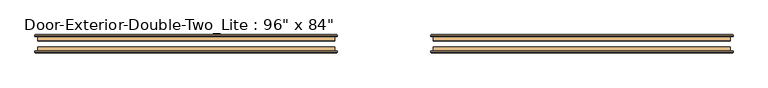
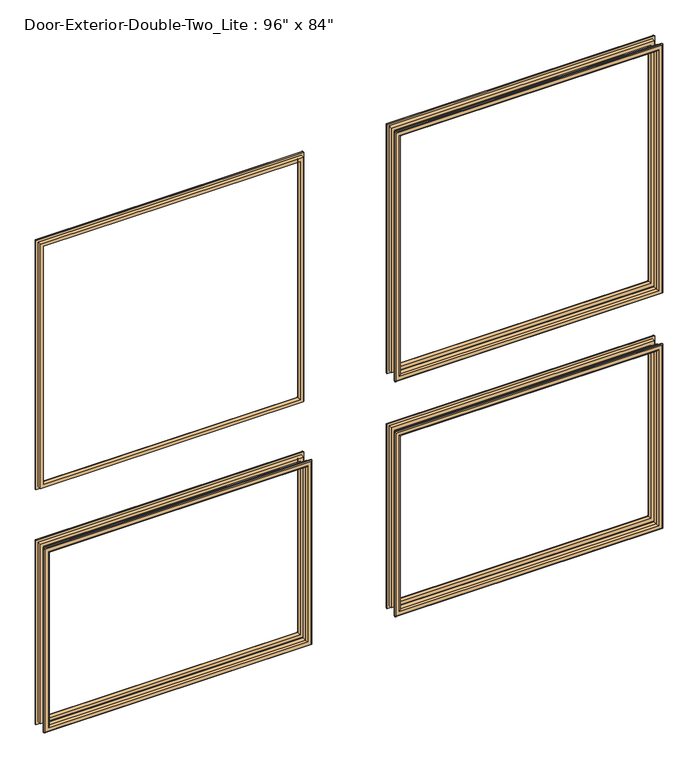
"""IFC4 building model written with IfcOpenShell, lengths in millimetres: door geometry."""

from ifc_helpers import new_model, si_unit, frame, origin, place, context, project, spatial, ellipse_curve, source, transform, mapped, element, save
from ifc_brep_helpers import plane_surface, cylinder_surface, advanced_brep


def door_142f3e8c(model_context):
    return source(origin(), model_context, "Body", "AdvancedBrep", [
        advanced_brep(
        [(-1066.8, 69.85, 914.4), (-1066.8, 82.55, 914.4), (-1066.8, 82.55, 254.0), (-1066.8, 69.85, 254.0), (-1054.8, 83.55, 902.4), (-1054.8, 69.85, 902.4), (-1054.8, 69.85, 266.0), (-1054.8, 83.55, 266.0), (-1059.8, 88.55, 907.4), (-1059.8, 88.55, 261.0), (-1074.8, 86.55, 922.4), (-1072.8, 88.55, 920.4), (-1072.8, 88.55, 248.0), (-1074.8, 86.55, 246.0), (-1074.8, 82.55, 922.4), (-1074.8, 82.55, 246.0), (-152.4, 82.55, 254.0), (-152.4, 69.85, 254.0), (-164.4, 69.85, 266.0), (-164.4, 83.55, 266.0), (-159.4, 88.55, 261.0), (-146.4, 88.55, 248.0), (-144.4, 86.55, 246.0), (-144.4, 82.55, 246.0), (-152.4, 82.55, 914.4), (-152.4, 69.85, 914.4), (-164.4, 69.85, 902.4), (-164.4, 83.55, 902.4), (-159.4, 88.55, 907.4), (-146.4, 88.55, 920.4), (-144.4, 86.55, 922.4), (-144.4, 82.55, 922.4)],
        [
            (0, 1),
            (1, 2),
            (2, 3),
            (3, 0),
            (4, 5),
            (5, 6),
            (6, 7),
            (7, 4),
            (8, 4, ellipse_curve(frame((-1059.8, 83.55, 907.4), z_axis=(-0.7071067811865475, 0.0, -0.7071067811865475), x_axis=(-0.7071067811865474, 0.0, 0.7071067811865476)), 7.0710678, 5.0)),
            (7, 9, ellipse_curve(frame((-1059.8, 83.55, 261.0), z_axis=(-0.7071067811865475, 0.0, 0.7071067811865475), x_axis=(0.7071067811865474, 0.0, 0.7071067811865476)), 7.0710678, 5.0)),
            (9, 8),
            (10, 11, ellipse_curve(frame((-1072.8, 86.55, 920.4), z_axis=(-0.7071067811865475, 0.0, -0.7071067811865475), x_axis=(-0.7071067811865474, 0.0, 0.7071067811865476)), 2.8284271, 2.0)),
            (11, 12),
            (12, 13, ellipse_curve(frame((-1072.8, 86.55, 248.0), z_axis=(-0.7071067811865475, 0.0, 0.7071067811865475), x_axis=(0.7071067811865474, 0.0, 0.7071067811865476)), 2.8284271, 2.0)),
            (13, 10),
            (14, 10),
            (13, 15),
            (15, 14),
            (2, 16),
            (16, 17),
            (17, 3),
            (6, 18),
            (18, 19),
            (19, 7),
            (19, 20, ellipse_curve(frame((-159.4, 83.55, 261.0), z_axis=(-0.7071067811865475, 0.0, -0.7071067811865475), x_axis=(-0.7071067811865476, 0.0, 0.7071067811865474)), 7.0710678, 5.0)),
            (20, 9),
            (12, 21),
            (21, 22, ellipse_curve(frame((-146.4, 86.55, 248.0), z_axis=(-0.7071067811865475, 0.0, -0.7071067811865475), x_axis=(-0.7071067811865476, 0.0, 0.7071067811865474)), 2.8284271, 2.0)),
            (22, 13),
            (22, 23),
            (23, 15),
            (16, 24),
            (24, 25),
            (25, 17),
            (18, 26),
            (26, 27),
            (27, 19),
            (27, 28, ellipse_curve(frame((-159.4, 83.55, 907.4), z_axis=(0.7071067811865475, 0.0, -0.7071067811865475), x_axis=(-0.7071067811865474, 0.0, -0.7071067811865476)), 7.0710678, 5.0)),
            (28, 20),
            (21, 29),
            (29, 30, ellipse_curve(frame((-146.4, 86.55, 920.4), z_axis=(0.7071067811865475, 0.0, -0.7071067811865475), x_axis=(-0.7071067811865474, 0.0, -0.7071067811865476)), 2.8284271, 2.0)),
            (30, 22),
            (30, 31),
            (31, 23),
            (31, 14),
            (1, 24),
            (0, 25),
            (5, 26),
            (4, 27),
            (8, 28),
            (11, 29),
            (10, 30),
        ],
        [
            plane_surface(frame((-1066.8, 82.55, 914.4), z_axis=(-1.0, 0.0, 0.0), x_axis=(0.0, 0.0, -1.0))),
            plane_surface(frame((-1054.8, 69.85, 902.4), z_axis=(1.0, 0.0, 0.0), x_axis=(0.0, 0.0, -1.0))),
            cylinder_surface(frame((-1059.8, 83.55, 914.4), z_axis=(0.0, 0.0, 1.0), x_axis=(-1.0, 0.0, 0.0)), 5.0),
            cylinder_surface(frame((-1072.8, 86.55, 914.4), z_axis=(0.0, 0.0, 1.0), x_axis=(-1.0, 0.0, 0.0)), 2.0),
            plane_surface(frame((-1074.8, 86.55, 922.4), z_axis=(-1.0, 0.0, 0.0), x_axis=(0.0, 0.0, -1.0))),
            plane_surface(frame((-1066.8, 82.55, 254.0), z_axis=(0.0, 0.0, -1.0), x_axis=(1.0, 0.0, 0.0))),
            plane_surface(frame((-1054.8, 69.85, 266.0), z_axis=(0.0, 0.0, 1.0), x_axis=(1.0, 0.0, 0.0))),
            cylinder_surface(frame((-1066.8, 83.55, 261.0), z_axis=(-1.0, 0.0, 0.0), x_axis=(0.0, 0.0, -1.0)), 5.0),
            cylinder_surface(frame((-1066.8, 86.55, 248.0), z_axis=(-1.0, 0.0, 0.0), x_axis=(0.0, 0.0, -1.0)), 2.0),
            plane_surface(frame((-1074.8, 86.55, 246.0), z_axis=(0.0, 0.0, -1.0), x_axis=(1.0, 0.0, 0.0))),
            plane_surface(frame((-152.4, 82.55, 254.0), z_axis=(1.0, 0.0, 0.0), x_axis=(0.0, 0.0, 1.0))),
            plane_surface(frame((-164.4, 69.85, 266.0), z_axis=(-1.0, 0.0, 0.0), x_axis=(0.0, 0.0, 1.0))),
            cylinder_surface(frame((-159.4, 83.55, 254.0), z_axis=(0.0, 0.0, -1.0), x_axis=(1.0, 0.0, 0.0)), 5.0),
            cylinder_surface(frame((-146.4, 86.55, 254.0), z_axis=(0.0, 0.0, -1.0), x_axis=(1.0, 0.0, 0.0)), 2.0),
            plane_surface(frame((-144.4, 86.55, 246.0), z_axis=(1.0, 0.0, 0.0), x_axis=(0.0, 0.0, 1.0))),
            plane_surface(frame((-144.4, 82.55, 922.4), z_axis=(0.0, -1.0, 0.0), x_axis=(-1.0, 0.0, 0.0))),
            plane_surface(frame((-152.4, 82.55, 914.4), z_axis=(0.0, 0.0, 1.0), x_axis=(-1.0, 0.0, 0.0))),
            plane_surface(frame((-152.4, 69.85, 914.4), z_axis=(0.0, -1.0, 0.0), x_axis=(-1.0, 0.0, 0.0))),
            plane_surface(frame((-164.4, 69.85, 902.4), z_axis=(0.0, 0.0, -1.0), x_axis=(-1.0, 0.0, 0.0))),
            cylinder_surface(frame((-152.4, 83.55, 907.4), z_axis=(1.0, 0.0, 0.0), x_axis=(0.0, 0.0, 1.0)), 5.0),
            plane_surface(frame((-159.4, 88.55, 907.4), z_axis=(0.0, 1.0, 0.0), x_axis=(-1.0, 0.0, 0.0))),
            cylinder_surface(frame((-152.4, 86.55, 920.4), z_axis=(1.0, 0.0, 0.0), x_axis=(0.0, 0.0, 1.0)), 2.0),
            plane_surface(frame((-144.4, 86.55, 922.4), z_axis=(0.0, 0.0, 1.0), x_axis=(-1.0, 0.0, 0.0))),
        ],
        [
            (0, [[1, 2, 3, 4]]),
            (1, [[5, 6, 7, 8]]),
            (2, [[9, -8, 10, 11]]),
            (3, [[12, 13, 14, 15]]),
            (4, [[16, -15, 17, 18]]),
            (5, [[-3, 19, 20, 21]]),
            (6, [[-7, 22, 23, 24]]),
            (7, [[-10, -24, 25, 26]]),
            (8, [[-14, 27, 28, 29]]),
            (9, [[-17, -29, 30, 31]]),
            (10, [[-20, 32, 33, 34]]),
            (11, [[-23, 35, 36, 37]]),
            (12, [[-25, -37, 38, 39]]),
            (13, [[-28, 40, 41, 42]]),
            (14, [[-30, -42, 43, 44]]),
            (15, [[-31, -44, 45, -18], [46, -32, -19, -2]]),
            (16, [[-33, -46, -1, 47]]),
            (17, [[-21, -34, -47, -4], [48, -35, -22, -6]]),
            (18, [[-36, -48, -5, 49]]),
            (19, [[-38, -49, -9, 50]]),
            (20, [[51, -40, -27, -13], [-26, -39, -50, -11]]),
            (21, [[-41, -51, -12, 52]]),
            (22, [[-43, -52, -16, -45]]),
        ],
    ),
        advanced_brep(
        [(152.4, 69.85, 914.4), (152.4, 82.55, 914.4), (152.4, 82.55, 254.0), (152.4, 69.85, 254.0), (164.4, 83.55, 902.4), (164.4, 69.85, 902.4), (164.4, 69.85, 266.0), (164.4, 83.55, 266.0), (159.4, 88.55, 907.4), (159.4, 88.55, 261.0), (144.4, 86.55, 922.4), (146.4, 88.55, 920.4), (146.4, 88.55, 248.0), (144.4, 86.55, 246.0), (144.4, 82.55, 922.4), (144.4, 82.55, 246.0), (1066.8, 82.55, 254.0), (1066.8, 69.85, 254.0), (1054.8, 69.85, 266.0), (1054.8, 83.55, 266.0), (1059.8, 88.55, 261.0), (1072.8, 88.55, 248.0), (1074.8, 86.55, 246.0), (1074.8, 82.55, 246.0), (1066.8, 82.55, 914.4), (1066.8, 69.85, 914.4), (1054.8, 69.85, 902.4), (1054.8, 83.55, 902.4), (1059.8, 88.55, 907.4), (1072.8, 88.55, 920.4), (1074.8, 86.55, 922.4), (1074.8, 82.55, 922.4)],
        [
            (0, 1),
            (1, 2),
            (2, 3),
            (3, 0),
            (4, 5),
            (5, 6),
            (6, 7),
            (7, 4),
            (8, 4, ellipse_curve(frame((159.4, 83.55, 907.4), z_axis=(-0.7071067811865475, 0.0, -0.7071067811865475), x_axis=(-0.7071067811865474, 0.0, 0.7071067811865476)), 7.0710678, 5.0)),
            (7, 9, ellipse_curve(frame((159.4, 83.55, 261.0), z_axis=(-0.7071067811865475, 0.0, 0.7071067811865475), x_axis=(0.7071067811865474, 0.0, 0.7071067811865476)), 7.0710678, 5.0)),
            (9, 8),
            (10, 11, ellipse_curve(frame((146.4, 86.55, 920.4), z_axis=(-0.7071067811865475, 0.0, -0.7071067811865475), x_axis=(-0.7071067811865474, 0.0, 0.7071067811865476)), 2.8284271, 2.0)),
            (11, 12),
            (12, 13, ellipse_curve(frame((146.4, 86.55, 248.0), z_axis=(-0.7071067811865475, 0.0, 0.7071067811865475), x_axis=(0.7071067811865474, 0.0, 0.7071067811865476)), 2.8284271, 2.0)),
            (13, 10),
            (14, 10),
            (13, 15),
            (15, 14),
            (2, 16),
            (16, 17),
            (17, 3),
            (6, 18),
            (18, 19),
            (19, 7),
            (19, 20, ellipse_curve(frame((1059.8, 83.55, 261.0), z_axis=(-0.7071067811865475, 0.0, -0.7071067811865475), x_axis=(-0.7071067811865476, 0.0, 0.7071067811865474)), 7.0710678, 5.0)),
            (20, 9),
            (12, 21),
            (21, 22, ellipse_curve(frame((1072.8, 86.55, 248.0), z_axis=(-0.7071067811865475, 0.0, -0.7071067811865475), x_axis=(-0.7071067811865476, 0.0, 0.7071067811865474)), 2.8284271, 2.0)),
            (22, 13),
            (22, 23),
            (23, 15),
            (16, 24),
            (24, 25),
            (25, 17),
            (18, 26),
            (26, 27),
            (27, 19),
            (27, 28, ellipse_curve(frame((1059.8, 83.55, 907.4), z_axis=(0.7071067811865475, 0.0, -0.7071067811865475), x_axis=(-0.7071067811865474, 0.0, -0.7071067811865476)), 7.0710678, 5.0)),
            (28, 20),
            (21, 29),
            (29, 30, ellipse_curve(frame((1072.8, 86.55, 920.4), z_axis=(0.7071067811865475, 0.0, -0.7071067811865475), x_axis=(-0.7071067811865474, 0.0, -0.7071067811865476)), 2.8284271, 2.0)),
            (30, 22),
            (30, 31),
            (31, 23),
            (31, 14),
            (1, 24),
            (0, 25),
            (5, 26),
            (4, 27),
            (8, 28),
            (11, 29),
            (10, 30),
        ],
        [
            plane_surface(frame((152.4, 82.55, 914.4), z_axis=(-1.0, 0.0, 0.0), x_axis=(0.0, 0.0, -1.0))),
            plane_surface(frame((164.4, 69.85, 902.4), z_axis=(1.0, 0.0, 0.0), x_axis=(0.0, 0.0, -1.0))),
            cylinder_surface(frame((159.4, 83.55, 914.4), z_axis=(0.0, 0.0, 1.0), x_axis=(-1.0, 0.0, 0.0)), 5.0),
            cylinder_surface(frame((146.4, 86.55, 914.4), z_axis=(0.0, 0.0, 1.0), x_axis=(-1.0, 0.0, 0.0)), 2.0),
            plane_surface(frame((144.4, 86.55, 922.4), z_axis=(-1.0, 0.0, 0.0), x_axis=(0.0, 0.0, -1.0))),
            plane_surface(frame((152.4, 82.55, 254.0), z_axis=(0.0, 0.0, -1.0), x_axis=(1.0, 0.0, 0.0))),
            plane_surface(frame((164.4, 69.85, 266.0), z_axis=(0.0, 0.0, 1.0), x_axis=(1.0, 0.0, 0.0))),
            cylinder_surface(frame((152.4, 83.55, 261.0), z_axis=(-1.0, 0.0, 0.0), x_axis=(0.0, 0.0, -1.0)), 5.0),
            cylinder_surface(frame((152.4, 86.55, 248.0), z_axis=(-1.0, 0.0, 0.0), x_axis=(0.0, 0.0, -1.0)), 2.0),
            plane_surface(frame((144.4, 86.55, 246.0), z_axis=(0.0, 0.0, -1.0), x_axis=(1.0, 0.0, 0.0))),
            plane_surface(frame((1066.8, 82.55, 254.0), z_axis=(1.0, 0.0, 0.0), x_axis=(0.0, 0.0, 1.0))),
            plane_surface(frame((1054.8, 69.85, 266.0), z_axis=(-1.0, 0.0, 0.0), x_axis=(0.0, 0.0, 1.0))),
            cylinder_surface(frame((1059.8, 83.55, 254.0), z_axis=(0.0, 0.0, -1.0), x_axis=(1.0, 0.0, 0.0)), 5.0),
            cylinder_surface(frame((1072.8, 86.55, 254.0), z_axis=(0.0, 0.0, -1.0), x_axis=(1.0, 0.0, 0.0)), 2.0),
            plane_surface(frame((1074.8, 86.55, 246.0), z_axis=(1.0, 0.0, 0.0), x_axis=(0.0, 0.0, 1.0))),
            plane_surface(frame((1074.8, 82.55, 922.4), z_axis=(0.0, -1.0, 0.0), x_axis=(-1.0, 0.0, 0.0))),
            plane_surface(frame((1066.8, 82.55, 914.4), z_axis=(0.0, 0.0, 1.0), x_axis=(-1.0, 0.0, 0.0))),
            plane_surface(frame((1066.8, 69.85, 914.4), z_axis=(0.0, -1.0, 0.0), x_axis=(-1.0, 0.0, 0.0))),
            plane_surface(frame((1054.8, 69.85, 902.4), z_axis=(0.0, 0.0, -1.0), x_axis=(-1.0, 0.0, 0.0))),
            cylinder_surface(frame((1066.8, 83.55, 907.4), z_axis=(1.0, 0.0, 0.0), x_axis=(0.0, 0.0, 1.0)), 5.0),
            plane_surface(frame((1059.8, 88.55, 907.4), z_axis=(0.0, 1.0, 0.0), x_axis=(-1.0, 0.0, 0.0))),
            cylinder_surface(frame((1066.8, 86.55, 920.4), z_axis=(1.0, 0.0, 0.0), x_axis=(0.0, 0.0, 1.0)), 2.0),
            plane_surface(frame((1074.8, 86.55, 922.4), z_axis=(0.0, 0.0, 1.0), x_axis=(-1.0, 0.0, 0.0))),
        ],
        [
            (0, [[1, 2, 3, 4]]),
            (1, [[5, 6, 7, 8]]),
            (2, [[9, -8, 10, 11]]),
            (3, [[12, 13, 14, 15]]),
            (4, [[16, -15, 17, 18]]),
            (5, [[-3, 19, 20, 21]]),
            (6, [[-7, 22, 23, 24]]),
            (7, [[-10, -24, 25, 26]]),
            (8, [[-14, 27, 28, 29]]),
            (9, [[-17, -29, 30, 31]]),
            (10, [[-20, 32, 33, 34]]),
            (11, [[-23, 35, 36, 37]]),
            (12, [[-25, -37, 38, 39]]),
            (13, [[-28, 40, 41, 42]]),
            (14, [[-30, -42, 43, 44]]),
            (15, [[-31, -44, 45, -18], [46, -32, -19, -2]]),
            (16, [[-33, -46, -1, 47]]),
            (17, [[-21, -34, -47, -4], [48, -35, -22, -6]]),
            (18, [[-36, -48, -5, 49]]),
            (19, [[-38, -49, -9, 50]]),
            (20, [[51, -40, -27, -13], [-26, -39, -50, -11]]),
            (21, [[-41, -51, -12, 52]]),
            (22, [[-43, -52, -16, -45]]),
        ],
    ),
        advanced_brep(
        [(152.4, 69.85, 2016.125), (152.4, 82.55, 2016.125), (152.4, 82.55, 1117.6), (152.4, 69.85, 1117.6), (164.4, 83.55, 2004.125), (164.4, 69.85, 2004.125), (164.4, 69.85, 1129.6), (164.4, 83.55, 1129.6), (159.4, 88.55, 2009.125), (159.4, 88.55, 1124.6), (144.4, 86.55, 2024.125), (146.4, 88.55, 2022.125), (146.4, 88.55, 1111.6), (144.4, 86.55, 1109.6), (144.4, 82.55, 2024.125), (144.4, 82.55, 1109.6), (1066.8, 82.55, 1117.6), (1066.8, 69.85, 1117.6), (1054.8, 69.85, 1129.6), (1054.8, 83.55, 1129.6), (1059.8, 88.55, 1124.6), (1072.8, 88.55, 1111.6), (1074.8, 86.55, 1109.6), (1074.8, 82.55, 1109.6), (1066.8, 82.55, 2016.125), (1066.8, 69.85, 2016.125), (1054.8, 69.85, 2004.125), (1054.8, 83.55, 2004.125), (1059.8, 88.55, 2009.125), (1072.8, 88.55, 2022.125), (1074.8, 86.55, 2024.125), (1074.8, 82.55, 2024.125)],
        [
            (0, 1),
            (1, 2),
            (2, 3),
            (3, 0),
            (4, 5),
            (5, 6),
            (6, 7),
            (7, 4),
            (8, 4, ellipse_curve(frame((159.4, 83.55, 2009.125), z_axis=(-0.7071067811865475, 0.0, -0.7071067811865475), x_axis=(-0.7071067811865474, 0.0, 0.7071067811865476)), 7.0710678, 5.0)),
            (7, 9, ellipse_curve(frame((159.4, 83.55, 1124.6), z_axis=(-0.7071067811865475, 0.0, 0.7071067811865475), x_axis=(0.7071067811865474, 0.0, 0.7071067811865476)), 7.0710678, 5.0)),
            (9, 8),
            (10, 11, ellipse_curve(frame((146.4, 86.55, 2022.125), z_axis=(-0.7071067811865475, 0.0, -0.7071067811865475), x_axis=(-0.7071067811865474, 0.0, 0.7071067811865476)), 2.8284271, 2.0)),
            (11, 12),
            (12, 13, ellipse_curve(frame((146.4, 86.55, 1111.6), z_axis=(-0.7071067811865475, 0.0, 0.7071067811865475), x_axis=(0.7071067811865474, 0.0, 0.7071067811865476)), 2.8284271, 2.0)),
            (13, 10),
            (14, 10),
            (13, 15),
            (15, 14),
            (2, 16),
            (16, 17),
            (17, 3),
            (6, 18),
            (18, 19),
            (19, 7),
            (19, 20, ellipse_curve(frame((1059.8, 83.55, 1124.6), z_axis=(-0.7071067811865475, 0.0, -0.7071067811865475), x_axis=(-0.7071067811865476, 0.0, 0.7071067811865474)), 7.0710678, 5.0)),
            (20, 9),
            (12, 21),
            (21, 22, ellipse_curve(frame((1072.8, 86.55, 1111.6), z_axis=(-0.7071067811865475, 0.0, -0.7071067811865475), x_axis=(-0.7071067811865476, 0.0, 0.7071067811865474)), 2.8284271, 2.0)),
            (22, 13),
            (22, 23),
            (23, 15),
            (16, 24),
            (24, 25),
            (25, 17),
            (18, 26),
            (26, 27),
            (27, 19),
            (27, 28, ellipse_curve(frame((1059.8, 83.55, 2009.125), z_axis=(0.7071067811865475, 0.0, -0.7071067811865475), x_axis=(-0.7071067811865474, 0.0, -0.7071067811865476)), 7.0710678, 5.0)),
            (28, 20),
            (21, 29),
            (29, 30, ellipse_curve(frame((1072.8, 86.55, 2022.125), z_axis=(0.7071067811865475, 0.0, -0.7071067811865475), x_axis=(-0.7071067811865474, 0.0, -0.7071067811865476)), 2.8284271, 2.0)),
            (30, 22),
            (30, 31),
            (31, 23),
            (31, 14),
            (1, 24),
            (0, 25),
            (5, 26),
            (4, 27),
            (8, 28),
            (11, 29),
            (10, 30),
        ],
        [
            plane_surface(frame((152.4, 82.55, 2016.125), z_axis=(-1.0, 0.0, 0.0), x_axis=(0.0, 0.0, -1.0))),
            plane_surface(frame((164.4, 69.85, 2004.125), z_axis=(1.0, 0.0, 0.0), x_axis=(0.0, 0.0, -1.0))),
            cylinder_surface(frame((159.4, 83.55, 2016.125), z_axis=(0.0, 0.0, 1.0), x_axis=(-1.0, 0.0, 0.0)), 5.0),
            cylinder_surface(frame((146.4, 86.55, 2016.125), z_axis=(0.0, 0.0, 1.0), x_axis=(-1.0, 0.0, 0.0)), 2.0),
            plane_surface(frame((144.4, 86.55, 2024.125), z_axis=(-1.0, 0.0, 0.0), x_axis=(0.0, 0.0, -1.0))),
            plane_surface(frame((152.4, 82.55, 1117.6), z_axis=(0.0, 0.0, -1.0), x_axis=(1.0, 0.0, 0.0))),
            plane_surface(frame((164.4, 69.85, 1129.6), z_axis=(0.0, 0.0, 1.0), x_axis=(1.0, 0.0, 0.0))),
            cylinder_surface(frame((152.4, 83.55, 1124.6), z_axis=(-1.0, 0.0, 0.0), x_axis=(0.0, 0.0, -1.0)), 5.0),
            cylinder_surface(frame((152.4, 86.55, 1111.6), z_axis=(-1.0, 0.0, 0.0), x_axis=(0.0, 0.0, -1.0)), 2.0),
            plane_surface(frame((144.4, 86.55, 1109.6), z_axis=(0.0, 0.0, -1.0), x_axis=(1.0, 0.0, 0.0))),
            plane_surface(frame((1066.8, 82.55, 1117.6), z_axis=(1.0, 0.0, 0.0), x_axis=(0.0, 0.0, 1.0))),
            plane_surface(frame((1054.8, 69.85, 1129.6), z_axis=(-1.0, 0.0, 0.0), x_axis=(0.0, 0.0, 1.0))),
            cylinder_surface(frame((1059.8, 83.55, 1117.6), z_axis=(0.0, 0.0, -1.0), x_axis=(1.0, 0.0, 0.0)), 5.0),
            cylinder_surface(frame((1072.8, 86.55, 1117.6), z_axis=(0.0, 0.0, -1.0), x_axis=(1.0, 0.0, 0.0)), 2.0),
            plane_surface(frame((1074.8, 86.55, 1109.6), z_axis=(1.0, 0.0, 0.0), x_axis=(0.0, 0.0, 1.0))),
            plane_surface(frame((1074.8, 82.55, 2024.125), z_axis=(0.0, -1.0, 0.0), x_axis=(-1.0, 0.0, 0.0))),
            plane_surface(frame((1066.8, 82.55, 2016.125), z_axis=(0.0, 0.0, 1.0), x_axis=(-1.0, 0.0, 0.0))),
            plane_surface(frame((1066.8, 69.85, 2016.125), z_axis=(0.0, -1.0, 0.0), x_axis=(-1.0, 0.0, 0.0))),
            plane_surface(frame((1054.8, 69.85, 2004.125), z_axis=(0.0, 0.0, -1.0), x_axis=(-1.0, 0.0, 0.0))),
            cylinder_surface(frame((1066.8, 83.55, 2009.125), z_axis=(1.0, 0.0, 0.0), x_axis=(0.0, 0.0, 1.0)), 5.0),
            plane_surface(frame((1059.8, 88.55, 2009.125), z_axis=(0.0, 1.0, 0.0), x_axis=(-1.0, 0.0, 0.0))),
            cylinder_surface(frame((1066.8, 86.55, 2022.125), z_axis=(1.0, 0.0, 0.0), x_axis=(0.0, 0.0, 1.0)), 2.0),
            plane_surface(frame((1074.8, 86.55, 2024.125), z_axis=(0.0, 0.0, 1.0), x_axis=(-1.0, 0.0, 0.0))),
        ],
        [
            (0, [[1, 2, 3, 4]]),
            (1, [[5, 6, 7, 8]]),
            (2, [[9, -8, 10, 11]]),
            (3, [[12, 13, 14, 15]]),
            (4, [[16, -15, 17, 18]]),
            (5, [[-3, 19, 20, 21]]),
            (6, [[-7, 22, 23, 24]]),
            (7, [[-10, -24, 25, 26]]),
            (8, [[-14, 27, 28, 29]]),
            (9, [[-17, -29, 30, 31]]),
            (10, [[-20, 32, 33, 34]]),
            (11, [[-23, 35, 36, 37]]),
            (12, [[-25, -37, 38, 39]]),
            (13, [[-28, 40, 41, 42]]),
            (14, [[-30, -42, 43, 44]]),
            (15, [[-31, -44, 45, -18], [46, -32, -19, -2]]),
            (16, [[-33, -46, -1, 47]]),
            (17, [[-21, -34, -47, -4], [48, -35, -22, -6]]),
            (18, [[-36, -48, -5, 49]]),
            (19, [[-38, -49, -9, 50]]),
            (20, [[51, -40, -27, -13], [-26, -39, -50, -11]]),
            (21, [[-41, -51, -12, 52]]),
            (22, [[-43, -52, -16, -45]]),
        ],
    ),
        advanced_brep(
        [(-1066.8, 69.85, 2016.125), (-1066.8, 82.55, 2016.125), (-1066.8, 82.55, 1117.6), (-1066.8, 69.85, 1117.6), (-1054.8, 83.55, 2004.125), (-1054.8, 69.85, 2004.125), (-1054.8, 69.85, 1129.6), (-1054.8, 83.55, 1129.6), (-1059.8, 88.55, 2009.125), (-1059.8, 88.55, 1124.6), (-1074.8, 86.55, 2024.125), (-1072.8, 88.55, 2022.125), (-1072.8, 88.55, 1111.6), (-1074.8, 86.55, 1109.6), (-1074.8, 82.55, 2024.125), (-1074.8, 82.55, 1109.6), (-152.4, 82.55, 1117.6), (-152.4, 69.85, 1117.6), (-164.4, 69.85, 1129.6), (-164.4, 83.55, 1129.6), (-159.4, 88.55, 1124.6), (-146.4, 88.55, 1111.6), (-144.4, 86.55, 1109.6), (-144.4, 82.55, 1109.6), (-152.4, 82.55, 2016.125), (-152.4, 69.85, 2016.125), (-164.4, 69.85, 2004.125), (-164.4, 83.55, 2004.125), (-159.4, 88.55, 2009.125), (-146.4, 88.55, 2022.125), (-144.4, 86.55, 2024.125), (-144.4, 82.55, 2024.125)],
        [
            (0, 1),
            (1, 2),
            (2, 3),
            (3, 0),
            (4, 5),
            (5, 6),
            (6, 7),
            (7, 4),
            (8, 4, ellipse_curve(frame((-1059.8, 83.55, 2009.125), z_axis=(-0.7071067811865475, 0.0, -0.7071067811865475), x_axis=(-0.7071067811865474, 0.0, 0.7071067811865476)), 7.0710678, 5.0)),
            (7, 9, ellipse_curve(frame((-1059.8, 83.55, 1124.6), z_axis=(-0.7071067811865475, 0.0, 0.7071067811865475), x_axis=(0.7071067811865474, 0.0, 0.7071067811865476)), 7.0710678, 5.0)),
            (9, 8),
            (10, 11, ellipse_curve(frame((-1072.8, 86.55, 2022.125), z_axis=(-0.7071067811865475, 0.0, -0.7071067811865475), x_axis=(-0.7071067811865474, 0.0, 0.7071067811865476)), 2.8284271, 2.0)),
            (11, 12),
            (12, 13, ellipse_curve(frame((-1072.8, 86.55, 1111.6), z_axis=(-0.7071067811865475, 0.0, 0.7071067811865475), x_axis=(0.7071067811865474, 0.0, 0.7071067811865476)), 2.8284271, 2.0)),
            (13, 10),
            (14, 10),
            (13, 15),
            (15, 14),
            (2, 16),
            (16, 17),
            (17, 3),
            (6, 18),
            (18, 19),
            (19, 7),
            (19, 20, ellipse_curve(frame((-159.4, 83.55, 1124.6), z_axis=(-0.7071067811865475, 0.0, -0.7071067811865475), x_axis=(-0.7071067811865476, 0.0, 0.7071067811865474)), 7.0710678, 5.0)),
            (20, 9),
            (12, 21),
            (21, 22, ellipse_curve(frame((-146.4, 86.55, 1111.6), z_axis=(-0.7071067811865475, 0.0, -0.7071067811865475), x_axis=(-0.7071067811865476, 0.0, 0.7071067811865474)), 2.8284271, 2.0)),
            (22, 13),
            (22, 23),
            (23, 15),
            (16, 24),
            (24, 25),
            (25, 17),
            (18, 26),
            (26, 27),
            (27, 19),
            (27, 28, ellipse_curve(frame((-159.4, 83.55, 2009.125), z_axis=(0.7071067811865475, 0.0, -0.7071067811865475), x_axis=(-0.7071067811865474, 0.0, -0.7071067811865476)), 7.0710678, 5.0)),
            (28, 20),
            (21, 29),
            (29, 30, ellipse_curve(frame((-146.4, 86.55, 2022.125), z_axis=(0.7071067811865475, 0.0, -0.7071067811865475), x_axis=(-0.7071067811865474, 0.0, -0.7071067811865476)), 2.8284271, 2.0)),
            (30, 22),
            (30, 31),
            (31, 23),
            (31, 14),
            (1, 24),
            (0, 25),
            (5, 26),
            (4, 27),
            (8, 28),
            (11, 29),
            (10, 30),
        ],
        [
            plane_surface(frame((-1066.8, 82.55, 2016.125), z_axis=(-1.0, 0.0, 0.0), x_axis=(0.0, 0.0, -1.0))),
            plane_surface(frame((-1054.8, 69.85, 2004.125), z_axis=(1.0, 0.0, 0.0), x_axis=(0.0, 0.0, -1.0))),
            cylinder_surface(frame((-1059.8, 83.55, 2016.125), z_axis=(0.0, 0.0, 1.0), x_axis=(-1.0, 0.0, 0.0)), 5.0),
            cylinder_surface(frame((-1072.8, 86.55, 2016.125), z_axis=(0.0, 0.0, 1.0), x_axis=(-1.0, 0.0, 0.0)), 2.0),
            plane_surface(frame((-1074.8, 86.55, 2024.125), z_axis=(-1.0, 0.0, 0.0), x_axis=(0.0, 0.0, -1.0))),
            plane_surface(frame((-1066.8, 82.55, 1117.6), z_axis=(0.0, 0.0, -1.0), x_axis=(1.0, 0.0, 0.0))),
            plane_surface(frame((-1054.8, 69.85, 1129.6), z_axis=(0.0, 0.0, 1.0), x_axis=(1.0, 0.0, 0.0))),
            cylinder_surface(frame((-1066.8, 83.55, 1124.6), z_axis=(-1.0, 0.0, 0.0), x_axis=(0.0, 0.0, -1.0)), 5.0),
            cylinder_surface(frame((-1066.8, 86.55, 1111.6), z_axis=(-1.0, 0.0, 0.0), x_axis=(0.0, 0.0, -1.0)), 2.0),
            plane_surface(frame((-1074.8, 86.55, 1109.6), z_axis=(0.0, 0.0, -1.0), x_axis=(1.0, 0.0, 0.0))),
            plane_surface(frame((-152.4, 82.55, 1117.6), z_axis=(1.0, 0.0, 0.0), x_axis=(0.0, 0.0, 1.0))),
            plane_surface(frame((-164.4, 69.85, 1129.6), z_axis=(-1.0, 0.0, 0.0), x_axis=(0.0, 0.0, 1.0))),
            cylinder_surface(frame((-159.4, 83.55, 1117.6), z_axis=(0.0, 0.0, -1.0), x_axis=(1.0, 0.0, 0.0)), 5.0),
            cylinder_surface(frame((-146.4, 86.55, 1117.6), z_axis=(0.0, 0.0, -1.0), x_axis=(1.0, 0.0, 0.0)), 2.0),
            plane_surface(frame((-144.4, 86.55, 1109.6), z_axis=(1.0, 0.0, 0.0), x_axis=(0.0, 0.0, 1.0))),
            plane_surface(frame((-144.4, 82.55, 2024.125), z_axis=(0.0, -1.0, 0.0), x_axis=(-1.0, 0.0, 0.0))),
            plane_surface(frame((-152.4, 82.55, 2016.125), z_axis=(0.0, 0.0, 1.0), x_axis=(-1.0, 0.0, 0.0))),
            plane_surface(frame((-152.4, 69.85, 2016.125), z_axis=(0.0, -1.0, 0.0), x_axis=(-1.0, 0.0, 0.0))),
            plane_surface(frame((-164.4, 69.85, 2004.125), z_axis=(0.0, 0.0, -1.0), x_axis=(-1.0, 0.0, 0.0))),
            cylinder_surface(frame((-152.4, 83.55, 2009.125), z_axis=(1.0, 0.0, 0.0), x_axis=(0.0, 0.0, 1.0)), 5.0),
            plane_surface(frame((-159.4, 88.55, 2009.125), z_axis=(0.0, 1.0, 0.0), x_axis=(-1.0, 0.0, 0.0))),
            cylinder_surface(frame((-152.4, 86.55, 2022.125), z_axis=(1.0, 0.0, 0.0), x_axis=(0.0, 0.0, 1.0)), 2.0),
            plane_surface(frame((-144.4, 86.55, 2024.125), z_axis=(0.0, 0.0, 1.0), x_axis=(-1.0, 0.0, 0.0))),
        ],
        [
            (0, [[1, 2, 3, 4]]),
            (1, [[5, 6, 7, 8]]),
            (2, [[9, -8, 10, 11]]),
            (3, [[12, 13, 14, 15]]),
            (4, [[16, -15, 17, 18]]),
            (5, [[-3, 19, 20, 21]]),
            (6, [[-7, 22, 23, 24]]),
            (7, [[-10, -24, 25, 26]]),
            (8, [[-14, 27, 28, 29]]),
            (9, [[-17, -29, 30, 31]]),
            (10, [[-20, 32, 33, 34]]),
            (11, [[-23, 35, 36, 37]]),
            (12, [[-25, -37, 38, 39]]),
            (13, [[-28, 40, 41, 42]]),
            (14, [[-30, -42, 43, 44]]),
            (15, [[-31, -44, 45, -18], [46, -32, -19, -2]]),
            (16, [[-33, -46, -1, 47]]),
            (17, [[-21, -34, -47, -4], [48, -35, -22, -6]]),
            (18, [[-36, -48, -5, 49]]),
            (19, [[-38, -49, -9, 50]]),
            (20, [[51, -40, -27, -13], [-26, -39, -50, -11]]),
            (21, [[-41, -51, -12, 52]]),
            (22, [[-43, -52, -16, -45]]),
        ],
    ),
        advanced_brep(
        [(-1066.8, 50.8, 254.0), (-1066.8, 38.1, 254.0), (-1066.8, 38.1, 914.4), (-1066.8, 50.8, 914.4), (-1054.8, 37.1, 266.0), (-1054.8, 50.8, 266.0), (-1054.8, 50.8, 902.4), (-1054.8, 37.1, 902.4), (-1059.8, 32.1, 261.0), (-1059.8, 32.1, 907.4), (-1074.8, 34.1, 246.0), (-1072.8, 32.1, 248.0), (-1072.8, 32.1, 920.4), (-1074.8, 34.1, 922.4), (-1074.8, 38.1, 246.0), (-1074.8, 38.1, 922.4), (-152.4, 38.1, 914.4), (-152.4, 50.8, 914.4), (-164.4, 50.8, 902.4), (-164.4, 37.1, 902.4), (-159.4, 32.1, 907.4), (-146.4, 32.1, 920.4), (-144.4, 34.1, 922.4), (-144.4, 38.1, 922.4), (-152.4, 38.1, 254.0), (-152.4, 50.8, 254.0), (-164.4, 50.8, 266.0), (-164.4, 37.1, 266.0), (-159.4, 32.1, 261.0), (-146.4, 32.1, 248.0), (-144.4, 34.1, 246.0), (-144.4, 38.1, 246.0)],
        [
            (0, 1),
            (1, 2),
            (2, 3),
            (3, 0),
            (4, 5),
            (5, 6),
            (6, 7),
            (7, 4),
            (8, 4, ellipse_curve(frame((-1059.8, 37.1, 261.0), z_axis=(-0.7071067811865475, 0.0, 0.7071067811865475), x_axis=(-0.7071067811865474, 0.0, -0.7071067811865476)), 7.0710678, 5.0)),
            (7, 9, ellipse_curve(frame((-1059.8, 37.1, 907.4), z_axis=(-0.7071067811865475, 0.0, -0.7071067811865475), x_axis=(0.7071067811865474, 0.0, -0.7071067811865476)), 7.0710678, 5.0)),
            (9, 8),
            (10, 11, ellipse_curve(frame((-1072.8, 34.1, 248.0), z_axis=(-0.7071067811865475, 0.0, 0.7071067811865475), x_axis=(-0.7071067811865474, 0.0, -0.7071067811865476)), 2.8284271, 2.0)),
            (11, 12),
            (12, 13, ellipse_curve(frame((-1072.8, 34.1, 920.4), z_axis=(-0.7071067811865475, 0.0, -0.7071067811865475), x_axis=(0.7071067811865474, 0.0, -0.7071067811865476)), 2.8284271, 2.0)),
            (13, 10),
            (14, 10),
            (13, 15),
            (15, 14),
            (2, 16),
            (16, 17),
            (17, 3),
            (6, 18),
            (18, 19),
            (19, 7),
            (19, 20, ellipse_curve(frame((-159.4, 37.1, 907.4), z_axis=(-0.7071067811865475, 0.0, 0.7071067811865475), x_axis=(-0.7071067811865476, 0.0, -0.7071067811865474)), 7.0710678, 5.0)),
            (20, 9),
            (12, 21),
            (21, 22, ellipse_curve(frame((-146.4, 34.1, 920.4), z_axis=(-0.7071067811865475, 0.0, 0.7071067811865475), x_axis=(-0.7071067811865476, 0.0, -0.7071067811865474)), 2.8284271, 2.0)),
            (22, 13),
            (22, 23),
            (23, 15),
            (16, 24),
            (24, 25),
            (25, 17),
            (18, 26),
            (26, 27),
            (27, 19),
            (27, 28, ellipse_curve(frame((-159.4, 37.1, 261.0), z_axis=(0.7071067811865475, 0.0, 0.7071067811865475), x_axis=(-0.7071067811865474, 0.0, 0.7071067811865476)), 7.0710678, 5.0)),
            (28, 20),
            (21, 29),
            (29, 30, ellipse_curve(frame((-146.4, 34.1, 248.0), z_axis=(0.7071067811865475, 0.0, 0.7071067811865475), x_axis=(-0.7071067811865474, 0.0, 0.7071067811865476)), 2.8284271, 2.0)),
            (30, 22),
            (30, 31),
            (31, 23),
            (31, 14),
            (1, 24),
            (0, 25),
            (5, 26),
            (4, 27),
            (8, 28),
            (11, 29),
            (10, 30),
        ],
        [
            plane_surface(frame((-1066.8, 38.1, 254.0), z_axis=(-1.0, 0.0, 0.0), x_axis=(0.0, 0.0, 1.0))),
            plane_surface(frame((-1054.8, 50.8, 266.0), z_axis=(1.0, 0.0, 0.0), x_axis=(0.0, 0.0, 1.0))),
            cylinder_surface(frame((-1059.8, 37.1, 254.0), z_axis=(0.0, 0.0, -1.0), x_axis=(-1.0, 0.0, 0.0)), 5.0),
            cylinder_surface(frame((-1072.8, 34.1, 254.0), z_axis=(0.0, 0.0, -1.0), x_axis=(-1.0, 0.0, 0.0)), 2.0),
            plane_surface(frame((-1074.8, 34.1, 246.0), z_axis=(-1.0, 0.0, 0.0), x_axis=(0.0, 0.0, 1.0))),
            plane_surface(frame((-1066.8, 38.1, 914.4), z_axis=(0.0, 0.0, 1.0), x_axis=(1.0, 0.0, 0.0))),
            plane_surface(frame((-1054.8, 50.8, 902.4), z_axis=(0.0, 0.0, -1.0), x_axis=(1.0, 0.0, 0.0))),
            cylinder_surface(frame((-1066.8, 37.1, 907.4), z_axis=(-1.0, 0.0, 0.0), x_axis=(0.0, 0.0, 1.0)), 5.0),
            cylinder_surface(frame((-1066.8, 34.1, 920.4), z_axis=(-1.0, 0.0, 0.0), x_axis=(0.0, 0.0, 1.0)), 2.0),
            plane_surface(frame((-1074.8, 34.1, 922.4), z_axis=(0.0, 0.0, 1.0), x_axis=(1.0, 0.0, 0.0))),
            plane_surface(frame((-152.4, 38.1, 914.4), z_axis=(1.0, 0.0, 0.0), x_axis=(0.0, 0.0, -1.0))),
            plane_surface(frame((-164.4, 50.8, 902.4), z_axis=(-1.0, 0.0, 0.0), x_axis=(0.0, 0.0, -1.0))),
            cylinder_surface(frame((-159.4, 37.1, 914.4), z_axis=(0.0, 0.0, 1.0), x_axis=(1.0, 0.0, 0.0)), 5.0),
            cylinder_surface(frame((-146.4, 34.1, 914.4), z_axis=(0.0, 0.0, 1.0), x_axis=(1.0, 0.0, 0.0)), 2.0),
            plane_surface(frame((-144.4, 34.1, 922.4), z_axis=(1.0, 0.0, 0.0), x_axis=(0.0, 0.0, -1.0))),
            plane_surface(frame((-144.4, 38.1, 246.0), z_axis=(0.0, 1.0, 0.0), x_axis=(-1.0, 0.0, 0.0))),
            plane_surface(frame((-152.4, 38.1, 254.0), z_axis=(0.0, 0.0, -1.0), x_axis=(-1.0, 0.0, 0.0))),
            plane_surface(frame((-152.4, 50.8, 254.0), z_axis=(0.0, 1.0, 0.0), x_axis=(-1.0, 0.0, 0.0))),
            plane_surface(frame((-164.4, 50.8, 266.0), z_axis=(0.0, 0.0, 1.0), x_axis=(-1.0, 0.0, 0.0))),
            cylinder_surface(frame((-152.4, 37.1, 261.0), z_axis=(1.0, 0.0, 0.0), x_axis=(0.0, 0.0, -1.0)), 5.0),
            plane_surface(frame((-159.4, 32.1, 261.0), z_axis=(0.0, -1.0, 0.0), x_axis=(-1.0, 0.0, 0.0))),
            cylinder_surface(frame((-152.4, 34.1, 248.0), z_axis=(1.0, 0.0, 0.0), x_axis=(0.0, 0.0, -1.0)), 2.0),
            plane_surface(frame((-144.4, 34.1, 246.0), z_axis=(0.0, 0.0, -1.0), x_axis=(-1.0, 0.0, 0.0))),
        ],
        [
            (0, [[1, 2, 3, 4]]),
            (1, [[5, 6, 7, 8]]),
            (2, [[9, -8, 10, 11]]),
            (3, [[12, 13, 14, 15]]),
            (4, [[16, -15, 17, 18]]),
            (5, [[-3, 19, 20, 21]]),
            (6, [[-7, 22, 23, 24]]),
            (7, [[-10, -24, 25, 26]]),
            (8, [[-14, 27, 28, 29]]),
            (9, [[-17, -29, 30, 31]]),
            (10, [[-20, 32, 33, 34]]),
            (11, [[-23, 35, 36, 37]]),
            (12, [[-25, -37, 38, 39]]),
            (13, [[-28, 40, 41, 42]]),
            (14, [[-30, -42, 43, 44]]),
            (15, [[-31, -44, 45, -18], [46, -32, -19, -2]]),
            (16, [[-33, -46, -1, 47]]),
            (17, [[-21, -34, -47, -4], [48, -35, -22, -6]]),
            (18, [[-36, -48, -5, 49]]),
            (19, [[-38, -49, -9, 50]]),
            (20, [[51, -40, -27, -13], [-26, -39, -50, -11]]),
            (21, [[-41, -51, -12, 52]]),
            (22, [[-43, -52, -16, -45]]),
        ],
    ),
        advanced_brep(
        [(152.4, 50.8, 254.0), (152.4, 38.1, 254.0), (152.4, 38.1, 914.4), (152.4, 50.8, 914.4), (164.4, 37.1, 266.0), (164.4, 50.8, 266.0), (164.4, 50.8, 902.4), (164.4, 37.1, 902.4), (159.4, 32.1, 261.0), (159.4, 32.1, 907.4), (144.4, 34.1, 246.0), (146.4, 32.1, 248.0), (146.4, 32.1, 920.4), (144.4, 34.1, 922.4), (144.4, 38.1, 246.0), (144.4, 38.1, 922.4), (1066.8, 38.1, 914.4), (1066.8, 50.8, 914.4), (1054.8, 50.8, 902.4), (1054.8, 37.1, 902.4), (1059.8, 32.1, 907.4), (1072.8, 32.1, 920.4), (1074.8, 34.1, 922.4), (1074.8, 38.1, 922.4), (1066.8, 38.1, 254.0), (1066.8, 50.8, 254.0), (1054.8, 50.8, 266.0), (1054.8, 37.1, 266.0), (1059.8, 32.1, 261.0), (1072.8, 32.1, 248.0), (1074.8, 34.1, 246.0), (1074.8, 38.1, 246.0)],
        [
            (0, 1),
            (1, 2),
            (2, 3),
            (3, 0),
            (4, 5),
            (5, 6),
            (6, 7),
            (7, 4),
            (8, 4, ellipse_curve(frame((159.4, 37.1, 261.0), z_axis=(-0.7071067811865475, 0.0, 0.7071067811865475), x_axis=(-0.7071067811865474, 0.0, -0.7071067811865476)), 7.0710678, 5.0)),
            (7, 9, ellipse_curve(frame((159.4, 37.1, 907.4), z_axis=(-0.7071067811865475, 0.0, -0.7071067811865475), x_axis=(0.7071067811865474, 0.0, -0.7071067811865476)), 7.0710678, 5.0)),
            (9, 8),
            (10, 11, ellipse_curve(frame((146.4, 34.1, 248.0), z_axis=(-0.7071067811865475, 0.0, 0.7071067811865475), x_axis=(-0.7071067811865474, 0.0, -0.7071067811865476)), 2.8284271, 2.0)),
            (11, 12),
            (12, 13, ellipse_curve(frame((146.4, 34.1, 920.4), z_axis=(-0.7071067811865475, 0.0, -0.7071067811865475), x_axis=(0.7071067811865474, 0.0, -0.7071067811865476)), 2.8284271, 2.0)),
            (13, 10),
            (14, 10),
            (13, 15),
            (15, 14),
            (2, 16),
            (16, 17),
            (17, 3),
            (6, 18),
            (18, 19),
            (19, 7),
            (19, 20, ellipse_curve(frame((1059.8, 37.1, 907.4), z_axis=(-0.7071067811865475, 0.0, 0.7071067811865475), x_axis=(-0.7071067811865476, 0.0, -0.7071067811865474)), 7.0710678, 5.0)),
            (20, 9),
            (12, 21),
            (21, 22, ellipse_curve(frame((1072.8, 34.1, 920.4), z_axis=(-0.7071067811865475, 0.0, 0.7071067811865475), x_axis=(-0.7071067811865476, 0.0, -0.7071067811865474)), 2.8284271, 2.0)),
            (22, 13),
            (22, 23),
            (23, 15),
            (16, 24),
            (24, 25),
            (25, 17),
            (18, 26),
            (26, 27),
            (27, 19),
            (27, 28, ellipse_curve(frame((1059.8, 37.1, 261.0), z_axis=(0.7071067811865475, 0.0, 0.7071067811865475), x_axis=(-0.7071067811865474, 0.0, 0.7071067811865476)), 7.0710678, 5.0)),
            (28, 20),
            (21, 29),
            (29, 30, ellipse_curve(frame((1072.8, 34.1, 248.0), z_axis=(0.7071067811865475, 0.0, 0.7071067811865475), x_axis=(-0.7071067811865474, 0.0, 0.7071067811865476)), 2.8284271, 2.0)),
            (30, 22),
            (30, 31),
            (31, 23),
            (31, 14),
            (1, 24),
            (0, 25),
            (5, 26),
            (4, 27),
            (8, 28),
            (11, 29),
            (10, 30),
        ],
        [
            plane_surface(frame((152.4, 38.1, 254.0), z_axis=(-1.0, 0.0, 0.0), x_axis=(0.0, 0.0, 1.0))),
            plane_surface(frame((164.4, 50.8, 266.0), z_axis=(1.0, 0.0, 0.0), x_axis=(0.0, 0.0, 1.0))),
            cylinder_surface(frame((159.4, 37.1, 254.0), z_axis=(0.0, 0.0, -1.0), x_axis=(-1.0, 0.0, 0.0)), 5.0),
            cylinder_surface(frame((146.4, 34.1, 254.0), z_axis=(0.0, 0.0, -1.0), x_axis=(-1.0, 0.0, 0.0)), 2.0),
            plane_surface(frame((144.4, 34.1, 246.0), z_axis=(-1.0, 0.0, 0.0), x_axis=(0.0, 0.0, 1.0))),
            plane_surface(frame((152.4, 38.1, 914.4), z_axis=(0.0, 0.0, 1.0), x_axis=(1.0, 0.0, 0.0))),
            plane_surface(frame((164.4, 50.8, 902.4), z_axis=(0.0, 0.0, -1.0), x_axis=(1.0, 0.0, 0.0))),
            cylinder_surface(frame((152.4, 37.1, 907.4), z_axis=(-1.0, 0.0, 0.0), x_axis=(0.0, 0.0, 1.0)), 5.0),
            cylinder_surface(frame((152.4, 34.1, 920.4), z_axis=(-1.0, 0.0, 0.0), x_axis=(0.0, 0.0, 1.0)), 2.0),
            plane_surface(frame((144.4, 34.1, 922.4), z_axis=(0.0, 0.0, 1.0), x_axis=(1.0, 0.0, 0.0))),
            plane_surface(frame((1066.8, 38.1, 914.4), z_axis=(1.0, 0.0, 0.0), x_axis=(0.0, 0.0, -1.0))),
            plane_surface(frame((1054.8, 50.8, 902.4), z_axis=(-1.0, 0.0, 0.0), x_axis=(0.0, 0.0, -1.0))),
            cylinder_surface(frame((1059.8, 37.1, 914.4), z_axis=(0.0, 0.0, 1.0), x_axis=(1.0, 0.0, 0.0)), 5.0),
            cylinder_surface(frame((1072.8, 34.1, 914.4), z_axis=(0.0, 0.0, 1.0), x_axis=(1.0, 0.0, 0.0)), 2.0),
            plane_surface(frame((1074.8, 34.1, 922.4), z_axis=(1.0, 0.0, 0.0), x_axis=(0.0, 0.0, -1.0))),
            plane_surface(frame((1074.8, 38.1, 246.0), z_axis=(0.0, 1.0, 0.0), x_axis=(-1.0, 0.0, 0.0))),
            plane_surface(frame((1066.8, 38.1, 254.0), z_axis=(0.0, 0.0, -1.0), x_axis=(-1.0, 0.0, 0.0))),
            plane_surface(frame((1066.8, 50.8, 254.0), z_axis=(0.0, 1.0, 0.0), x_axis=(-1.0, 0.0, 0.0))),
            plane_surface(frame((1054.8, 50.8, 266.0), z_axis=(0.0, 0.0, 1.0), x_axis=(-1.0, 0.0, 0.0))),
            cylinder_surface(frame((1066.8, 37.1, 261.0), z_axis=(1.0, 0.0, 0.0), x_axis=(0.0, 0.0, -1.0)), 5.0),
            plane_surface(frame((1059.8, 32.1, 261.0), z_axis=(0.0, -1.0, 0.0), x_axis=(-1.0, 0.0, 0.0))),
            cylinder_surface(frame((1066.8, 34.1, 248.0), z_axis=(1.0, 0.0, 0.0), x_axis=(0.0, 0.0, -1.0)), 2.0),
            plane_surface(frame((1074.8, 34.1, 246.0), z_axis=(0.0, 0.0, -1.0), x_axis=(-1.0, 0.0, 0.0))),
        ],
        [
            (0, [[1, 2, 3, 4]]),
            (1, [[5, 6, 7, 8]]),
            (2, [[9, -8, 10, 11]]),
            (3, [[12, 13, 14, 15]]),
            (4, [[16, -15, 17, 18]]),
            (5, [[-3, 19, 20, 21]]),
            (6, [[-7, 22, 23, 24]]),
            (7, [[-10, -24, 25, 26]]),
            (8, [[-14, 27, 28, 29]]),
            (9, [[-17, -29, 30, 31]]),
            (10, [[-20, 32, 33, 34]]),
            (11, [[-23, 35, 36, 37]]),
            (12, [[-25, -37, 38, 39]]),
            (13, [[-28, 40, 41, 42]]),
            (14, [[-30, -42, 43, 44]]),
            (15, [[-31, -44, 45, -18], [46, -32, -19, -2]]),
            (16, [[-33, -46, -1, 47]]),
            (17, [[-21, -34, -47, -4], [48, -35, -22, -6]]),
            (18, [[-36, -48, -5, 49]]),
            (19, [[-38, -49, -9, 50]]),
            (20, [[51, -40, -27, -13], [-26, -39, -50, -11]]),
            (21, [[-41, -51, -12, 52]]),
            (22, [[-43, -52, -16, -45]]),
        ],
    ),
        advanced_brep(
        [(152.4, 50.8, 1117.6), (152.4, 38.1, 1117.6), (152.4, 38.1, 2016.125), (152.4, 50.8, 2016.125), (164.4, 37.1, 1129.6), (164.4, 50.8, 1129.6), (164.4, 50.8, 2004.125), (164.4, 37.1, 2004.125), (159.4, 32.1, 1124.6), (159.4, 32.1, 2009.125), (144.4, 34.1, 1109.6), (146.4, 32.1, 1111.6), (146.4, 32.1, 2022.125), (144.4, 34.1, 2024.125), (144.4, 38.1, 1109.6), (144.4, 38.1, 2024.125), (1066.8, 38.1, 2016.125), (1066.8, 50.8, 2016.125), (1054.8, 50.8, 2004.125), (1054.8, 37.1, 2004.125), (1059.8, 32.1, 2009.125), (1072.8, 32.1, 2022.125), (1074.8, 34.1, 2024.125), (1074.8, 38.1, 2024.125), (1066.8, 38.1, 1117.6), (1066.8, 50.8, 1117.6), (1054.8, 50.8, 1129.6), (1054.8, 37.1, 1129.6), (1059.8, 32.1, 1124.6), (1072.8, 32.1, 1111.6), (1074.8, 34.1, 1109.6), (1074.8, 38.1, 1109.6)],
        [
            (0, 1),
            (1, 2),
            (2, 3),
            (3, 0),
            (4, 5),
            (5, 6),
            (6, 7),
            (7, 4),
            (8, 4, ellipse_curve(frame((159.4, 37.1, 1124.6), z_axis=(-0.7071067811865475, 0.0, 0.7071067811865475), x_axis=(-0.7071067811865474, 0.0, -0.7071067811865476)), 7.0710678, 5.0)),
            (7, 9, ellipse_curve(frame((159.4, 37.1, 2009.125), z_axis=(-0.7071067811865475, 0.0, -0.7071067811865475), x_axis=(0.7071067811865474, 0.0, -0.7071067811865476)), 7.0710678, 5.0)),
            (9, 8),
            (10, 11, ellipse_curve(frame((146.4, 34.1, 1111.6), z_axis=(-0.7071067811865475, 0.0, 0.7071067811865475), x_axis=(-0.7071067811865474, 0.0, -0.7071067811865476)), 2.8284271, 2.0)),
            (11, 12),
            (12, 13, ellipse_curve(frame((146.4, 34.1, 2022.125), z_axis=(-0.7071067811865475, 0.0, -0.7071067811865475), x_axis=(0.7071067811865474, 0.0, -0.7071067811865476)), 2.8284271, 2.0)),
            (13, 10),
            (14, 10),
            (13, 15),
            (15, 14),
            (2, 16),
            (16, 17),
            (17, 3),
            (6, 18),
            (18, 19),
            (19, 7),
            (19, 20, ellipse_curve(frame((1059.8, 37.1, 2009.125), z_axis=(-0.7071067811865475, 0.0, 0.7071067811865475), x_axis=(-0.7071067811865476, 0.0, -0.7071067811865474)), 7.0710678, 5.0)),
            (20, 9),
            (12, 21),
            (21, 22, ellipse_curve(frame((1072.8, 34.1, 2022.125), z_axis=(-0.7071067811865475, 0.0, 0.7071067811865475), x_axis=(-0.7071067811865476, 0.0, -0.7071067811865474)), 2.8284271, 2.0)),
            (22, 13),
            (22, 23),
            (23, 15),
            (16, 24),
            (24, 25),
            (25, 17),
            (18, 26),
            (26, 27),
            (27, 19),
            (27, 28, ellipse_curve(frame((1059.8, 37.1, 1124.6), z_axis=(0.7071067811865475, 0.0, 0.7071067811865475), x_axis=(-0.7071067811865474, 0.0, 0.7071067811865476)), 7.0710678, 5.0)),
            (28, 20),
            (21, 29),
            (29, 30, ellipse_curve(frame((1072.8, 34.1, 1111.6), z_axis=(0.7071067811865475, 0.0, 0.7071067811865475), x_axis=(-0.7071067811865474, 0.0, 0.7071067811865476)), 2.8284271, 2.0)),
            (30, 22),
            (30, 31),
            (31, 23),
            (31, 14),
            (1, 24),
            (0, 25),
            (5, 26),
            (4, 27),
            (8, 28),
            (11, 29),
            (10, 30),
        ],
        [
            plane_surface(frame((152.4, 38.1, 1117.6), z_axis=(-1.0, 0.0, 0.0), x_axis=(0.0, 0.0, 1.0))),
            plane_surface(frame((164.4, 50.8, 1129.6), z_axis=(1.0, 0.0, 0.0), x_axis=(0.0, 0.0, 1.0))),
            cylinder_surface(frame((159.4, 37.1, 1117.6), z_axis=(0.0, 0.0, -1.0), x_axis=(-1.0, 0.0, 0.0)), 5.0),
            cylinder_surface(frame((146.4, 34.1, 1117.6), z_axis=(0.0, 0.0, -1.0), x_axis=(-1.0, 0.0, 0.0)), 2.0),
            plane_surface(frame((144.4, 34.1, 1109.6), z_axis=(-1.0, 0.0, 0.0), x_axis=(0.0, 0.0, 1.0))),
            plane_surface(frame((152.4, 38.1, 2016.125), z_axis=(0.0, 0.0, 1.0), x_axis=(1.0, 0.0, 0.0))),
            plane_surface(frame((164.4, 50.8, 2004.125), z_axis=(0.0, 0.0, -1.0), x_axis=(1.0, 0.0, 0.0))),
            cylinder_surface(frame((152.4, 37.1, 2009.125), z_axis=(-1.0, 0.0, 0.0), x_axis=(0.0, 0.0, 1.0)), 5.0),
            cylinder_surface(frame((152.4, 34.1, 2022.125), z_axis=(-1.0, 0.0, 0.0), x_axis=(0.0, 0.0, 1.0)), 2.0),
            plane_surface(frame((144.4, 34.1, 2024.125), z_axis=(0.0, 0.0, 1.0), x_axis=(1.0, 0.0, 0.0))),
            plane_surface(frame((1066.8, 38.1, 2016.125), z_axis=(1.0, 0.0, 0.0), x_axis=(0.0, 0.0, -1.0))),
            plane_surface(frame((1054.8, 50.8, 2004.125), z_axis=(-1.0, 0.0, 0.0), x_axis=(0.0, 0.0, -1.0))),
            cylinder_surface(frame((1059.8, 37.1, 2016.125), z_axis=(0.0, 0.0, 1.0), x_axis=(1.0, 0.0, 0.0)), 5.0),
            cylinder_surface(frame((1072.8, 34.1, 2016.125), z_axis=(0.0, 0.0, 1.0), x_axis=(1.0, 0.0, 0.0)), 2.0),
            plane_surface(frame((1074.8, 34.1, 2024.125), z_axis=(1.0, 0.0, 0.0), x_axis=(0.0, 0.0, -1.0))),
            plane_surface(frame((1074.8, 38.1, 1109.6), z_axis=(0.0, 1.0, 0.0), x_axis=(-1.0, 0.0, 0.0))),
            plane_surface(frame((1066.8, 38.1, 1117.6), z_axis=(0.0, 0.0, -1.0), x_axis=(-1.0, 0.0, 0.0))),
            plane_surface(frame((1066.8, 50.8, 1117.6), z_axis=(0.0, 1.0, 0.0), x_axis=(-1.0, 0.0, 0.0))),
            plane_surface(frame((1054.8, 50.8, 1129.6), z_axis=(0.0, 0.0, 1.0), x_axis=(-1.0, 0.0, 0.0))),
            cylinder_surface(frame((1066.8, 37.1, 1124.6), z_axis=(1.0, 0.0, 0.0), x_axis=(0.0, 0.0, -1.0)), 5.0),
            plane_surface(frame((1059.8, 32.1, 1124.6), z_axis=(0.0, -1.0, 0.0), x_axis=(-1.0, 0.0, 0.0))),
            cylinder_surface(frame((1066.8, 34.1, 1111.6), z_axis=(1.0, 0.0, 0.0), x_axis=(0.0, 0.0, -1.0)), 2.0),
            plane_surface(frame((1074.8, 34.1, 1109.6), z_axis=(0.0, 0.0, -1.0), x_axis=(-1.0, 0.0, 0.0))),
        ],
        [
            (0, [[1, 2, 3, 4]]),
            (1, [[5, 6, 7, 8]]),
            (2, [[9, -8, 10, 11]]),
            (3, [[12, 13, 14, 15]]),
            (4, [[16, -15, 17, 18]]),
            (5, [[-3, 19, 20, 21]]),
            (6, [[-7, 22, 23, 24]]),
            (7, [[-10, -24, 25, 26]]),
            (8, [[-14, 27, 28, 29]]),
            (9, [[-17, -29, 30, 31]]),
            (10, [[-20, 32, 33, 34]]),
            (11, [[-23, 35, 36, 37]]),
            (12, [[-25, -37, 38, 39]]),
            (13, [[-28, 40, 41, 42]]),
            (14, [[-30, -42, 43, 44]]),
            (15, [[-31, -44, 45, -18], [46, -32, -19, -2]]),
            (16, [[-33, -46, -1, 47]]),
            (17, [[-21, -34, -47, -4], [48, -35, -22, -6]]),
            (18, [[-36, -48, -5, 49]]),
            (19, [[-38, -49, -9, 50]]),
            (20, [[51, -40, -27, -13], [-26, -39, -50, -11]]),
            (21, [[-41, -51, -12, 52]]),
            (22, [[-43, -52, -16, -45]]),
        ],
    ),
    ])


if __name__ == "__main__":
    model = new_model("IFC4")
    model_context = context("Model", 3, world=origin())
    ifc_project = project(units=[si_unit("LENGTHUNIT", "METRE", prefix="MILLI")], contexts=[model_context])
    site = spatial("IfcSite", under=ifc_project)
    building = spatial("IfcBuilding", under=site)
    placement = place(None, origin())
    door_shape = door_142f3e8c(model_context)
    element("IfcDoor", 1, ObjectType="Door-Exterior-Double-Two_Lite : 96\" x 84\"", at=placement, inside=building, context=model_context, shape_type="MappedRepresentation", body=[
        mapped(door_shape, transform((0.0, 0.0, 0.0), x_axis=(1.0, 0.0, 0.0), y_axis=(0.0, 1.0, 0.0), z_axis=(0.0, 0.0, 1.0))),
    ])
    save(model, "model.ifc")

# Revit data of these elements
# Type "Door-Exterior-Double-Two_Lite : 96\" x 84\""
#   Type Mark = "8"
#   Assembly Code = "B2030100"
#   Analytic Construction = "Metal frame, double glass door"
#   Top Rail = 0' - 4 5/8"
#   Threshold Length [instance default] = 8' - 4"
#   Threshold Offset [instance default] = 0' - 0 1/2"
#   Thickness = 0' - 1 3/4"
#   Thermal Resistance (R) = 1.3794 (h·ft²·°F)/BTU
#   Swing Angle [instance default] = 90.00°
#   Strike Height = 3' - 4"
#   Stiles = 0' - 6"
#   SinglePanelWidth = 4' - 0"
#   Rough Width [instance default] = 8' - 4"
#   Rough Height [instance default] = 7' - 4"
#   MFOpeningHeight [instance default] = 0' - 4"
#   MFOpeningWidth [instance default] = 0' - 4"
#   Lock Rail = 0' - 8"
#   Inset Calculate [instance default] = 0' - 4"
#   Masonry Inset [instance default] = 0' - 1"
#   Height = 7' - 0"
#   Width = 8' - 0"
#   Heat Transfer Coefficient (U) = 0.7250 BTU/(h·ft²·°F)
#   Glass Thickness = 0' - 0 3/4"
#   Masonry Frame Depth = 0' - 5 3/4"
#   Bottom Rail = 0' - 10"
#   Threshold [instance default] = yes
#   Masonry Frame [instance default] = yes
#   Wall Closure = 3
#   Function = 1
#   Dry Wall Frame [instance default] = no
#   Threshold Material = none
#   Panic Bar Material = Metal - Stainless Steel
#   Panel Material = Metal - Painted - Grey
#   Glass Stop Material = Metal - Painted - Grey
#   Frame Material = Metal - Painted - Grey
#   Exterior Pull Material = Metal - Stainless Steel
#   Visual Light Transmittance = 0
#   Solar Heat Gain Coefficient = 0
# Element 1 (IfcDoor, "Door-Exterior-Double-Two_Lite : 96\" x 84\"")
#   Materials on its faces: "Metal - Painted - Grey", "Metal - Stainless Steel", "Glass"
# Materials
#   "Metal - Stainless Steel": class "Metal", colour RGB 247 247 247, transparency 0
#   "Metal - Painted - Grey": class "Paint", colour RGB 104 104 104, transparency 0, Cost = 0
#   "Glass": class "Glass", colour RGB 0 128 192, transparency 0.75, Description = "Soda Lime Glass", Cost = 0
